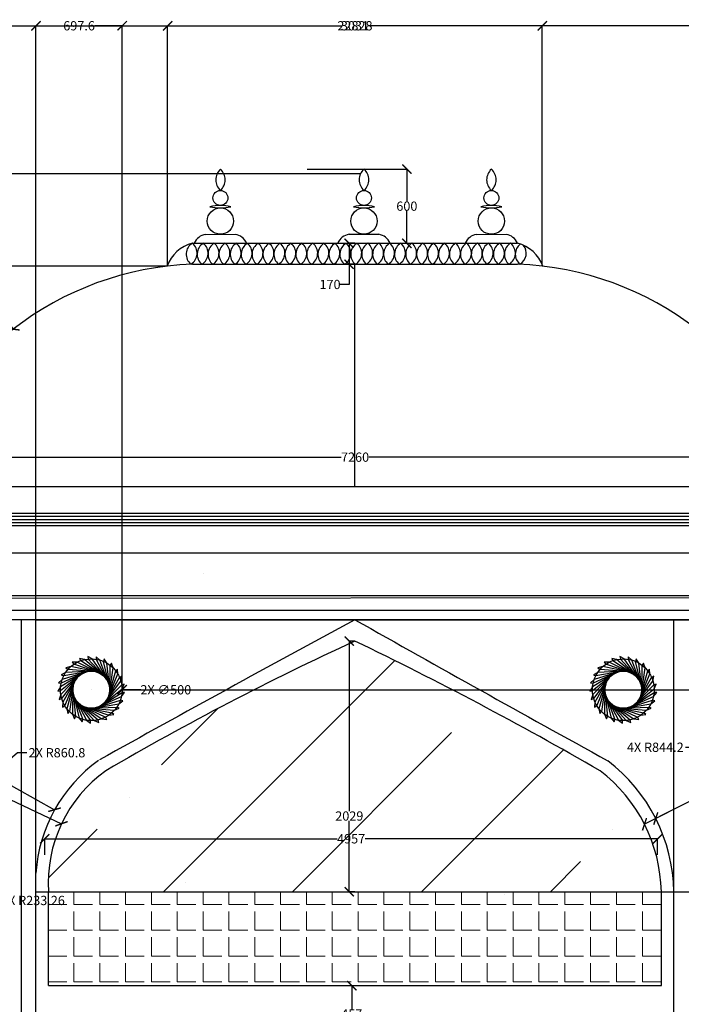
# Model space of a CAD drawing. Units: inches. Extents: x 829 to 33356404, y 1874 to 16983.
# Tile 7 of 9: x 10848 to 16199, y 9014 to 16983. Entities that reach past the tile are written whole.
import ezdxf

# ---------------------------------------------------------------- set-up
doc = ezdxf.new("R2010")
doc.units = ezdxf.units.IN
doc.header["$MEASUREMENT"] = 0
doc.header["$PDMODE"] = 3
for name, color, linetype, lineweight in [('A-ANNO-DIMS', 2, 'Continuous', 18), ('A-ELEV', 7, 'Continuous', 25), ('A-ELEV-PATT', 8, 'Continuous', 13)]:
    doc.layers.add(name, color=color, linetype=linetype, lineweight=lineweight)
doc.styles.get("Standard").update_dxf_attribs({"font": 'arial.ttf'})
doc.dimstyles.get("Standard").update_dxf_attribs({"dimtxt": 75, "dimasz": 75, "dimexe": 0.18, "dimexo": 0.0625, "dimgap": 0.09, "dimtad": 0, "dimtih": 1, "dimtoh": 1, "dimdec": 0, "dimzin": 0, "dimdsep": 46, "dimtxsty": 'Standard', "dimblk": 'ARCHTICK', "dimcen": 0.09, "dimadec": 0, "dimazin": 0, "dimtfac": 1, "dimtdec": 0, "dimtofl": 0, "dimtmove": 0, "dimatfit": 3, "dimfxl": 1, "dimtolj": 1, "dimtzin": 0, "dimarcsym": 0})

# ---------------------------------------------------------------- blocks, each defined once
blk = doc.blocks.new('_ArchTick')
at = {"color": 0, "linetype": 'ByBlock', "const_width": 0.15}
blk.add_lwpolyline([(-0.5, -0.5), (0.5, 0.5)], dxfattribs=at)
blk = doc.blocks.new('*D22')
at = {"layer": 'A-ANNO-DIMS', "color": 0, "lineweight": -2, "transparency": 16777216}
for p, q in [((13559.7, 11954.5), (13513.9, 11954.5)), ((13514.1, 11954.5), (13514.1, 10576.7)), ((13514.1, 9925.5), (13514.1, 10500)), ((13559.7, 9925.5), (13513.9, 9925.5))]:
    blk.add_line(p, q, dxfattribs=at)
at = {"layer": 'Defpoints', "color": 0, "transparency": 16777216}
for p in [(13514.1, 11954.5), (13559.8, 11954.5), (13559.8, 9925.5)]:
    blk.add_point(p, dxfattribs=at)
at = {"layer": 'A-ANNO-DIMS', "color": 0, "lineweight": -2, "transparency": 16777216, "xscale": 75, "yscale": 75, "zscale": 75}
for p, rotation in [((13514.1, 11954.5), 90), ((13514.1, 9925.5), 270)]:
    blk.add_blockref('_ArchTick', p, dxfattribs=dict(at, rotation=rotation))
at = {"layer": 'A-ANNO-DIMS', "color": 0, "transparency": 16777216, "insert": (13514.1, 10538.4), "char_height": 75, "attachment_point": 5}
blk.add_mtext('\\A1;2029', dxfattribs=at)
blk = doc.blocks.new('*D23')
at = {"layer": 'A-ANNO-DIMS', "color": 0, "lineweight": -2, "transparency": 16777216}
for p, q in [((11050.4, 10222.8), (11050.4, 10354.2)), ((11050.4, 10354), (13415.3, 10354)), ((16007.4, 10354), (13642.4, 10354)), ((16007.4, 10222.8), (16007.4, 10354.2))]:
    blk.add_line(p, q, dxfattribs=at)
at = {"layer": 'Defpoints', "color": 0, "transparency": 16777216}
for p in [(16007.4, 10354), (11050.4, 10222.7), (16007.4, 10222.7)]:
    blk.add_point(p, dxfattribs=at)
at = {"layer": 'A-ANNO-DIMS', "color": 0, "lineweight": -2, "transparency": 16777216, "xscale": 75, "yscale": 75, "zscale": 75, "rotation": 180}
blk.add_blockref('_ArchTick', (11050.4, 10354), dxfattribs=at)
at = {"layer": 'A-ANNO-DIMS', "color": 0, "lineweight": -2, "transparency": 16777216, "xscale": 75, "yscale": 75, "zscale": 75}
blk.add_blockref('_ArchTick', (16007.4, 10354), dxfattribs=at)
at = {"layer": 'A-ANNO-DIMS', "color": 0, "transparency": 16777216, "insert": (13528.9, 10354), "char_height": 75, "attachment_point": 5}
blk.add_mtext('\\A1;4957', dxfattribs=at)
blk = doc.blocks.new('*D24')
at = {"layer": 'A-ANNO-DIMS', "color": 0, "lineweight": -2, "transparency": 16777216}
for p, q in [((13534.6, 9165.5), (13534.3, 9165.5)), ((13534.5, 9165.5), (13534.5, 8975.2)), ((13534.5, 8708.5), (13534.5, 8898.7)), ((13534.6, 8708.5), (13534.3, 8708.5))]:
    blk.add_line(p, q, dxfattribs=at)
at = {"layer": 'Defpoints', "color": 0, "transparency": 16777216}
for p in [(13534.7, 9165.5), (13534.5, 8708.5), (13534.7, 8708.5)]:
    blk.add_point(p, dxfattribs=at)
at = {"layer": 'A-ANNO-DIMS', "color": 0, "lineweight": -2, "transparency": 16777216, "xscale": 75, "yscale": 75, "zscale": 75}
for p, rotation in [((13534.5, 9165.5), 90), ((13534.5, 8708.5), 270)]:
    blk.add_blockref('_ArchTick', p, dxfattribs=dict(at, rotation=rotation))
at = {"layer": 'A-ANNO-DIMS', "color": 0, "transparency": 16777216, "insert": (13534.5, 8937), "char_height": 75, "attachment_point": 5}
blk.add_mtext('\\A1;457', dxfattribs=at)
blk = doc.blocks.new('*D55')
at = {"layer": 'A-ANNO-DIMS', "color": 0, "lineweight": -2, "transparency": 16777216}
for p, q in [((9930.8, 13204.1), (9930.8, 13443)), ((9930.8, 13442.8), (13449.1, 13442.8)), ((17190.8, 13442.8), (13672.4, 13442.8)), ((17190.8, 13204.1), (17190.8, 13443))]:
    blk.add_line(p, q, dxfattribs=at)
at = {"layer": 'Defpoints', "color": 0, "transparency": 16777216}
for p in [(17190.8, 13442.8), (9930.8, 13204), (17190.8, 13204)]:
    blk.add_point(p, dxfattribs=at)
at = {"layer": 'A-ANNO-DIMS', "color": 0, "lineweight": -2, "transparency": 16777216, "xscale": 75, "yscale": 75, "zscale": 75, "rotation": 180}
blk.add_blockref('_ArchTick', (9930.8, 13442.8), dxfattribs=at)
at = {"layer": 'A-ANNO-DIMS', "color": 0, "lineweight": -2, "transparency": 16777216, "xscale": 75, "yscale": 75, "zscale": 75}
blk.add_blockref('_ArchTick', (17190.8, 13442.8), dxfattribs=at)
at = {"layer": 'A-ANNO-DIMS', "color": 0, "transparency": 16777216, "insert": (13560.8, 13442.8), "char_height": 75, "attachment_point": 5}
blk.add_mtext('\\A1;7260', dxfattribs=at)
blk = doc.blocks.new('*D56')
at = {"layer": 'A-ANNO-DIMS', "color": 0, "lineweight": -2, "transparency": 16777216}
for p, q in [((13559.7, 15174), (13512.5, 15174)), ((13512.7, 15174), (13512.7, 15004)), ((13559.7, 15004), (13512.5, 15004)), ((13512.7, 15004), (13512.7, 14840.3)), ((13512.7, 14840.3), (13437.7, 14840.3))]:
    blk.add_line(p, q, dxfattribs=at)
at = {"layer": 'Defpoints', "color": 0, "transparency": 16777216}
for p in [(13559.8, 15174), (13512.7, 15004), (13559.8, 15004)]:
    blk.add_point(p, dxfattribs=at)
at = {"layer": 'A-ANNO-DIMS', "color": 0, "lineweight": -2, "transparency": 16777216, "xscale": 75, "yscale": 75, "zscale": 75}
for p, rotation in [((13512.7, 15174), 90), ((13512.7, 15004), 270)]:
    blk.add_blockref('_ArchTick', p, dxfattribs=dict(at, rotation=rotation))
at = {"layer": 'A-ANNO-DIMS', "color": 0, "transparency": 16777216, "insert": (13358.4, 14840.3), "char_height": 75, "attachment_point": 5}
blk.add_mtext('\\A1;170', dxfattribs=at)
blk = doc.blocks.new('*D67')
at = {"layer": 'A-ANNO-DIMS', "color": 0, "lineweight": -2, "transparency": 16777216}
for p, q in [((13174.2, 15774), (13979.7, 15774)), ((13979.5, 15774), (13979.5, 15512.4)), ((13979.5, 15174), (13979.5, 15435.6)), ((13174.2, 15174), (13979.7, 15174))]:
    blk.add_line(p, q, dxfattribs=at)
at = {"layer": 'Defpoints', "color": 0, "transparency": 16777216}
for p in [(13174.2, 15774), (13979.5, 15774), (13174.2, 15174)]:
    blk.add_point(p, dxfattribs=at)
at = {"layer": 'A-ANNO-DIMS', "color": 0, "lineweight": -2, "transparency": 16777216, "xscale": 75, "yscale": 75, "zscale": 75}
for p, rotation in [((13979.5, 15774), 90), ((13979.5, 15174), 270)]:
    blk.add_blockref('_ArchTick', p, dxfattribs=dict(at, rotation=rotation))
at = {"layer": 'A-ANNO-DIMS', "color": 0, "transparency": 16777216, "insert": (13979.5, 15474), "char_height": 75, "attachment_point": 5}
blk.add_mtext('\\A1;600', dxfattribs=at)
blk = doc.blocks.new('*D82')
at = {"layer": 'A-ANNO-DIMS', "color": 0, "lineweight": -2, "transparency": 16777216}
for p, q in [((2145.7, 12292.3), (2145.7, 16934.2)), ((2145.7, 16934), (13417.9, 16934)), ((24973.9, 16934), (13701.7, 16934)), ((24973.9, 12320.9), (24973.9, 16934.2))]:
    blk.add_line(p, q, dxfattribs=at)
at = {"layer": 'Defpoints', "color": 0, "transparency": 16777216}
for p in [(24973.9, 16934), (2145.7, 12292.2), (24973.9, 12320.9)]:
    blk.add_point(p, dxfattribs=at)
at = {"layer": 'A-ANNO-DIMS', "color": 0, "lineweight": -2, "transparency": 16777216, "xscale": 75, "yscale": 75, "zscale": 75, "rotation": 180}
blk.add_blockref('_ArchTick', (2145.7, 16934), dxfattribs=at)
at = {"layer": 'A-ANNO-DIMS', "color": 0, "lineweight": -2, "transparency": 16777216, "xscale": 75, "yscale": 75, "zscale": 75}
blk.add_blockref('_ArchTick', (24973.9, 16934), dxfattribs=at)
at = {"layer": 'A-ANNO-DIMS', "color": 0, "transparency": 16777216, "insert": (13559.8, 16934), "char_height": 75, "attachment_point": 5}
blk.add_mtext('\\A1;22828', dxfattribs=at)
blk = doc.blocks.new('*D83')
at = {"layer": 'A-ANNO-DIMS', "color": 0, "lineweight": -2, "transparency": 16777216}
for p, q in [((13604.5, 15734.9), (985.4, 15734.9)), ((985.6, 15734.9), (985.6, 10279.1)), ((985.6, 4746.5), (985.6, 10202.3)), ((3169.7, 4746.5), (985.4, 4746.5))]:
    blk.add_line(p, q, dxfattribs=at)
at = {"layer": 'Defpoints', "color": 0, "transparency": 16777216}
for p in [(985.6, 15734.9), (13604.5, 15734.9), (3169.8, 4746.5)]:
    blk.add_point(p, dxfattribs=at)
at = {"layer": 'A-ANNO-DIMS', "color": 0, "lineweight": -2, "transparency": 16777216, "xscale": 75, "yscale": 75, "zscale": 75}
for p, rotation in [((985.6, 15734.9), 90), ((985.6, 4746.5), 270)]:
    blk.add_blockref('_ArchTick', p, dxfattribs=dict(at, rotation=rotation))
at = {"layer": 'A-ANNO-DIMS', "color": 0, "transparency": 16777216, "insert": (985.6, 10240.7), "char_height": 75, "attachment_point": 5}
blk.add_mtext('\\A1;10988', dxfattribs=at)
blk = doc.blocks.new('*D84')
at = {"layer": 'A-ANNO-DIMS', "color": 0, "lineweight": -2, "transparency": 16777216}
for p, q in [((12044.3, 14988.9), (985.4, 14988.9)), ((985.6, 14988.9), (985.6, 14134.8)), ((985.6, 13204), (985.6, 14058.1)), ((9930.7, 13204), (985.4, 13204))]:
    blk.add_line(p, q, dxfattribs=at)
at = {"layer": 'Defpoints', "color": 0, "transparency": 16777216}
for p in [(985.6, 14988.9), (12044.4, 14988.9), (9930.8, 13204)]:
    blk.add_point(p, dxfattribs=at)
at = {"layer": 'A-ANNO-DIMS', "color": 0, "lineweight": -2, "transparency": 16777216, "xscale": 75, "yscale": 75, "zscale": 75}
for p, rotation in [((985.6, 14988.9), 90), ((985.6, 13204), 270)]:
    blk.add_blockref('_ArchTick', p, dxfattribs=dict(at, rotation=rotation))
at = {"layer": 'A-ANNO-DIMS', "color": 0, "transparency": 16777216, "insert": (985.6, 14096.5), "char_height": 75, "attachment_point": 5}
blk.add_mtext('\\A1;1785', dxfattribs=at)
blk = doc.blocks.new('*D85')
at = {"layer": 'A-ANNO-DIMS', "color": 0, "lineweight": -2, "transparency": 16777216}
for p, q in [((12044.4, 14989), (12044.4, 16934.2)), ((12044.4, 16934), (13455, 16934)), ((15075.2, 16934), (13664.6, 16934)), ((15075.2, 14989), (15075.2, 16934.2))]:
    blk.add_line(p, q, dxfattribs=at)
at = {"layer": 'Defpoints', "color": 0, "transparency": 16777216}
for p in [(15075.2, 16934), (12044.4, 14988.9), (15075.2, 14988.9)]:
    blk.add_point(p, dxfattribs=at)
at = {"layer": 'A-ANNO-DIMS', "color": 0, "lineweight": -2, "transparency": 16777216, "xscale": 75, "yscale": 75, "zscale": 75, "rotation": 180}
blk.add_blockref('_ArchTick', (12044.4, 16934), dxfattribs=at)
at = {"layer": 'A-ANNO-DIMS', "color": 0, "lineweight": -2, "transparency": 16777216, "xscale": 75, "yscale": 75, "zscale": 75}
blk.add_blockref('_ArchTick', (15075.2, 16934), dxfattribs=at)
at = {"layer": 'A-ANNO-DIMS', "color": 0, "transparency": 16777216, "insert": (13559.8, 16934), "char_height": 75, "attachment_point": 5}
blk.add_mtext('\\A1;3031', dxfattribs=at)
blk = doc.blocks.new('*D91')
at = {"layer": 'A-ANNO-DIMS', "color": 0, "lineweight": -2, "transparency": 16777216}
for p, q in [((11081.8, 9925.5), (26134.1, 9925.5)), ((26133.9, 9925.5), (26133.9, 9354.7)), ((26133.9, 8708.5), (26133.9, 9279.2)), ((11081.8, 8708.5), (26134.1, 8708.5))]:
    blk.add_line(p, q, dxfattribs=at)
at = {"layer": 'Defpoints', "color": 0, "transparency": 16777216}
for p in [(11081.8, 9925.5), (11081.8, 8708.5), (26133.9, 8708.5)]:
    blk.add_point(p, dxfattribs=at)
at = {"layer": 'A-ANNO-DIMS', "color": 0, "lineweight": -2, "transparency": 16777216, "xscale": 75, "yscale": 75, "zscale": 75}
for p, rotation in [((26133.9, 9925.5), 90), ((26133.9, 8708.5), 270)]:
    blk.add_blockref('_ArchTick', p, dxfattribs=dict(at, rotation=rotation))
at = {"layer": 'A-ANNO-DIMS', "color": 0, "transparency": 16777216, "insert": (26133.9, 9317), "char_height": 75, "attachment_point": 5}
blk.add_mtext('\\A1;1217', dxfattribs=at)
blk = doc.blocks.new('*D92')
at = {"layer": 'A-ANNO-DIMS', "color": 0, "lineweight": -2, "transparency": 16777216}
for p, q in [((10979.8, 12127.3), (10979.8, 16934.2)), ((10979.8, 16934), (11201.8, 16934)), ((11677.4, 16934), (11455.4, 16934)), ((11677.4, 11560.1), (11677.4, 16934.2))]:
    blk.add_line(p, q, dxfattribs=at)
at = {"layer": 'Defpoints', "color": 0, "transparency": 16777216}
for p in [(11677.4, 16934), (10979.8, 12127.2), (11677.4, 11560.1)]:
    blk.add_point(p, dxfattribs=at)
at = {"layer": 'A-ANNO-DIMS', "color": 0, "lineweight": -2, "transparency": 16777216, "xscale": 75, "yscale": 75, "zscale": 75, "rotation": 180}
blk.add_blockref('_ArchTick', (10979.8, 16934), dxfattribs=at)
at = {"layer": 'A-ANNO-DIMS', "color": 0, "lineweight": -2, "transparency": 16777216, "xscale": 75, "yscale": 75, "zscale": 75}
blk.add_blockref('_ArchTick', (11677.4, 16934), dxfattribs=at)
at = {"layer": 'A-ANNO-DIMS', "color": 0, "transparency": 16777216, "insert": (11328.6, 16934), "char_height": 75, "attachment_point": 5}
blk.add_mtext('\\A1;697.6', dxfattribs=at)
blk = doc.blocks.new('*D93')
at = {"layer": 'A-ANNO-DIMS', "color": 0, "lineweight": -2, "transparency": 16777216}
for p, q in [((10979.8, 12127.2), (26134.1, 12127.2)), ((26133.9, 12127.2), (26133.9, 11882)), ((26133.9, 11560.1), (26133.9, 11805.3)), ((11677.4, 11560.1), (26134.1, 11560.1))]:
    blk.add_line(p, q, dxfattribs=at)
at = {"layer": 'Defpoints', "color": 0, "transparency": 16777216}
for p in [(10979.8, 12127.2), (11677.4, 11560.1), (26133.9, 11560.1)]:
    blk.add_point(p, dxfattribs=at)
at = {"layer": 'A-ANNO-DIMS', "color": 0, "lineweight": -2, "transparency": 16777216, "xscale": 75, "yscale": 75, "zscale": 75}
for p, rotation in [((26133.9, 12127.2), 90), ((26133.9, 11560.1), 270)]:
    blk.add_blockref('_ArchTick', p, dxfattribs=dict(at, rotation=rotation))
at = {"layer": 'A-ANNO-DIMS', "color": 0, "transparency": 16777216, "insert": (26133.9, 11843.6), "char_height": 75, "attachment_point": 5}
blk.add_mtext('\\A1;567.1', dxfattribs=at)
blk = doc.blocks.new('*D109')
at = {"layer": 'A-ANNO-DIMS', "color": 0, "lineweight": -2, "transparency": 16777216}
for p, q in [((9798.3, 15665.5), (9873.3, 15665.5)), ((9873.3, 15665.5), (10796, 14478.3)), ((12333.6, 12499.6), (12333.8, 12499.6)), ((12333.7, 12499.5), (12333.7, 12499.7))]:
    blk.add_line(p, q, dxfattribs=at)
at = {"layer": 'Defpoints', "color": 0, "transparency": 16777216}
for p in [(10796, 14478.3), (12333.7, 12499.6)]:
    blk.add_point(p, dxfattribs=at)
at = {"layer": 'A-ANNO-DIMS', "color": 0, "lineweight": -2, "transparency": 16777216, "xscale": 75, "yscale": 75, "zscale": 75, "rotation": 307.8527471709181}
blk.add_blockref('_ArchTick', (10796, 14478.3), dxfattribs=at)
at = {"layer": 'A-ANNO-DIMS', "color": 0, "transparency": 16777216, "insert": (9569.2, 15665.5), "char_height": 75, "attachment_point": 5}
blk.add_mtext('\\A1;2X R2506', dxfattribs=at)
blk = doc.blocks.new('*D123')
at = {"layer": 'A-ANNO-DIMS', "color": 0, "lineweight": -2, "transparency": 16777216}
for p, q in [((10418.6, 10943.5), (10493.6, 10943.5)), ((10493.6, 10943.5), (11130.3, 10589.5)), ((12191.3, 9999.5), (12191.5, 9999.5)), ((12191.4, 9999.4), (12191.4, 9999.6))]:
    blk.add_line(p, q, dxfattribs=at)
at = {"layer": 'Defpoints', "color": 0, "transparency": 16777216}
for p in [(11130.3, 10589.5), (12191.4, 9999.5)]:
    blk.add_point(p, dxfattribs=at)
at = {"layer": 'A-ANNO-DIMS', "color": 0, "lineweight": -2, "transparency": 16777216, "xscale": 75, "yscale": 75, "zscale": 75, "rotation": 330.9254937916661}
blk.add_blockref('_ArchTick', (11130.3, 10589.5), dxfattribs=at)
at = {"layer": 'A-ANNO-DIMS', "color": 0, "transparency": 16777216, "insert": (10270.8, 10943.5), "char_height": 75, "attachment_point": 5}
blk.add_mtext('\\A1;R1214', dxfattribs=at)
blk = doc.blocks.new('*D124')
at = {"layer": 'A-ANNO-DIMS', "color": 0, "lineweight": -2, "transparency": 16777216}
for p, q in [((10508.3, 10761.1), (10583.3, 10761.1)), ((10583.3, 10761.1), (11186.3, 10475.5)), ((12191.3, 9999.5), (12191.5, 9999.5)), ((12191.4, 9999.4), (12191.4, 9999.6))]:
    blk.add_line(p, q, dxfattribs=at)
at = {"layer": 'Defpoints', "color": 0, "transparency": 16777216}
for p in [(11186.3, 10475.5), (12191.4, 9999.5)]:
    blk.add_point(p, dxfattribs=at)
at = {"layer": 'A-ANNO-DIMS', "color": 0, "lineweight": -2, "transparency": 16777216, "xscale": 75, "yscale": 75, "zscale": 75, "rotation": 334.6586083454434}
blk.add_blockref('_ArchTick', (11186.3, 10475.5), dxfattribs=at)
at = {"layer": 'A-ANNO-DIMS', "color": 0, "transparency": 16777216, "insert": (10323.9, 10761.1), "char_height": 75, "attachment_point": 5}
blk.add_mtext('\\A1;R1112.1', dxfattribs=at)
blk = doc.blocks.new('*D125')
at = {"layer": 'A-ANNO-DIMS', "color": 0, "lineweight": -2, "transparency": 16777216}
for p, q in [((16724.8, 10888.3), (15992.6, 10517.8)), ((16799.8, 10888.3), (16724.8, 10888.3)), ((14772.3, 9900.1), (14772.5, 9900.1)), ((14772.4, 9900), (14772.4, 9900.2))]:
    blk.add_line(p, q, dxfattribs=at)
at = {"layer": 'Defpoints', "color": 0, "transparency": 16777216}
for p in [(15992.6, 10517.8), (14772.4, 9900.1)]:
    blk.add_point(p, dxfattribs=at)
at = {"layer": 'A-ANNO-DIMS', "color": 0, "lineweight": -2, "transparency": 16777216, "xscale": 75, "yscale": 75, "zscale": 75, "rotation": 206.8466405163161}
blk.add_blockref('_ArchTick', (15992.6, 10517.8), dxfattribs=at)
at = {"layer": 'A-ANNO-DIMS', "color": 0, "transparency": 16777216, "insert": (16991.4, 10888.3), "char_height": 75, "attachment_point": 5}
blk.add_mtext('\\A1;R1367.6', dxfattribs=at)
blk = doc.blocks.new('*D126')
at = {"layer": 'A-ANNO-DIMS', "color": 0, "lineweight": -2, "transparency": 16777216}
for p, q in [((16579.1, 10814.6), (15901.6, 10471.7)), ((16654.1, 10814.6), (16579.1, 10814.6)), ((14772.3, 9900.1), (14772.5, 9900.1)), ((14772.4, 9900), (14772.4, 9900.2))]:
    blk.add_line(p, q, dxfattribs=at)
at = {"layer": 'Defpoints', "color": 0, "transparency": 16777216}
for p in [(15901.6, 10471.7), (14772.4, 9900.1)]:
    blk.add_point(p, dxfattribs=at)
at = {"layer": 'A-ANNO-DIMS', "color": 0, "lineweight": -2, "transparency": 16777216, "xscale": 75, "yscale": 75, "zscale": 75, "rotation": 206.8466187545911}
blk.add_blockref('_ArchTick', (15901.6, 10471.7), dxfattribs=at)
at = {"layer": 'A-ANNO-DIMS', "color": 0, "transparency": 16777216, "insert": (16845.8, 10814.6), "char_height": 75, "attachment_point": 5}
blk.add_mtext('\\A1;R1265.6', dxfattribs=at)
blk = doc.blocks.new('*D127')
at = {"layer": 'A-ANNO-DIMS', "color": 0, "lineweight": -2, "transparency": 16777216}
for p, q in [((11427.3, 11560.1), (11427.5, 11560.1)), ((11427.4, 11560), (11427.4, 11560.2)), ((11827.4, 11560.1), (11677.4, 11560.1))]:
    blk.add_line(p, q, dxfattribs=at)
at = {"layer": 'Defpoints', "color": 0, "transparency": 16777216}
for p in [(11177.4, 11560.1), (11677.4, 11560.1)]:
    blk.add_point(p, dxfattribs=at)
at = {"layer": 'A-ANNO-DIMS', "color": 0, "lineweight": -2, "transparency": 16777216, "xscale": 75, "yscale": 75, "zscale": 75, "rotation": 180.0000873187677}
blk.add_blockref('_ArchTick', (11677.4, 11560.1), dxfattribs=at)
at = {"layer": 'A-ANNO-DIMS', "color": 0, "transparency": 16777216, "insert": (12030.2, 11560.1), "char_height": 75, "attachment_point": 5}
blk.add_mtext('\\A1;2X ∅500', dxfattribs=at)
blk = doc.blocks.new('*D129')
at = {"layer": 'A-ANNO-DIMS', "color": 0, "lineweight": -2, "transparency": 16777216}
for p, q in [((10830.9, 11050.5), (10439.6, 10713.3)), ((10905.9, 11050.5), (10830.9, 11050.5)), ((9787.3, 10151.5), (9787.5, 10151.5)), ((9787.4, 10151.4), (9787.4, 10151.6))]:
    blk.add_line(p, q, dxfattribs=at)
at = {"layer": 'Defpoints', "color": 0, "transparency": 16777216}
for p in [(10439.6, 10713.3), (9787.4, 10151.5)]:
    blk.add_point(p, dxfattribs=at)
at = {"layer": 'A-ANNO-DIMS', "color": 0, "lineweight": -2, "transparency": 16777216, "xscale": 75, "yscale": 75, "zscale": 75, "rotation": 220.7456490042762}
blk.add_blockref('_ArchTick', (10439.6, 10713.3), dxfattribs=at)
at = {"layer": 'A-ANNO-DIMS', "color": 0, "transparency": 16777216, "insert": (11149.7, 11050.5), "char_height": 75, "attachment_point": 5}
blk.add_mtext('\\A1;2X R860.8', dxfattribs=at)
blk = doc.blocks.new('*D130')
at = {"layer": 'A-ANNO-DIMS', "color": 0, "lineweight": -2, "transparency": 16777216}
for p, q in [((16233.3, 11094.9), (16308.3, 11094.9)), ((16308.3, 11094.9), (16682.6, 10753.6)), ((17306.3, 10184.7), (17306.5, 10184.7)), ((17306.4, 10184.6), (17306.4, 10184.8))]:
    blk.add_line(p, q, dxfattribs=at)
at = {"layer": 'Defpoints', "color": 0, "transparency": 16777216}
for p in [(16682.6, 10753.6), (17306.4, 10184.7)]:
    blk.add_point(p, dxfattribs=at)
at = {"layer": 'A-ANNO-DIMS', "color": 0, "lineweight": -2, "transparency": 16777216, "xscale": 75, "yscale": 75, "zscale": 75, "rotation": 317.6357309782866}
blk.add_blockref('_ArchTick', (16682.6, 10753.6), dxfattribs=at)
at = {"layer": 'A-ANNO-DIMS', "color": 0, "transparency": 16777216, "insert": (15989.1, 11094.9), "char_height": 75, "attachment_point": 5}
blk.add_mtext('\\A1;4X R844.2', dxfattribs=at)
blk = doc.blocks.new('*D134')
at = {"layer": 'A-ANNO-DIMS', "color": 0, "lineweight": -2, "transparency": 16777216}
for p, q in [((10607.7, 9854.8), (10543.8, 9719.1)), ((10682.7, 9854.8), (10607.7, 9854.8)), ((10444.4, 9508.1), (10444.5, 9508.1)), ((10444.5, 9508), (10444.5, 9508.2))]:
    blk.add_line(p, q, dxfattribs=at)
at = {"layer": 'Defpoints', "color": 0, "transparency": 16777216}
for p in [(10543.8, 9719.1), (10444.5, 9508.1)]:
    blk.add_point(p, dxfattribs=at)
at = {"layer": 'A-ANNO-DIMS', "color": 0, "lineweight": -2, "transparency": 16777216, "xscale": 75, "yscale": 75, "zscale": 75, "rotation": 244.7886305373675}
blk.add_blockref('_ArchTick', (10543.8, 9719.1), dxfattribs=at)
at = {"layer": 'A-ANNO-DIMS', "color": 0, "transparency": 16777216, "insert": (10955.6, 9854.8), "char_height": 75, "attachment_point": 5}
blk.add_mtext('\\A1;2X R233.26', dxfattribs=at)

msp = doc.modelspace()

# ---------------------------------------------------------------- hatches: boundary and pattern name
at = {"layer": 'A-ELEV-PATT'}
h = msp.add_hatch(dxfattribs=at)
h.set_pattern_fill('ANSI35', color=256, scale=5900)
h.paths.add_polyline_path([(13559.778, 11954.468, 0.02477271), (11545.586, 10904.83, 0.26007445), (11081.778, 9925.468), (16037.778, 9925.468, 0.22810939), (15542.066, 10904.83, 0.01846983)])
h.paths.add_polyline_path([(13379.549, 10460.544), (13650.132, 10460.544), (13650.132, 10615.097), (13379.549, 10615.097)], flags=24)
h.paths.add_polyline_path([(13395.284, 10276.184), (13665.867, 10276.184), (13665.867, 10430.737), (13395.284, 10430.737)], flags=24)
h = msp.add_hatch(dxfattribs=at)
h.set_pattern_fill('ANGLE', color=256, scale=760)
h.set_pattern_definition([(0, (0, 0), (0, 209), [152, -57]), (90, (0, 0), (-209, 1e-14), [152, -57])])
h.paths.add_polyline_path([(11081.778, 9925.468), (11081.778, 9165.468), (16037.778, 9165.468), (16037.778, 9925.468)])

# ---------------------------------------------------------------- linework, layer by layer
at = {"layer": 'A-ELEV'}
for p, q in [((12351.34, 15245.971), (12591.591, 15247.24)), ((13512.395, 15246.139), (13752.646, 15247.408)), ((14542.78, 15245.971), (14783.031, 15247.24)), ((12244.919, 15174.032), (14874.638, 15174.032)), ((12244.919, 15004.032), (14874.638, 15004.032)), ((13559.778, 13204.032), (13559.778, 15004.032)), ((3169.778, 13204.032), (23949.778, 13204.032)), ((23949.778, 12986.532), (3169.778, 12986.532)), ((23949.778, 12961.532), (3169.778, 12961.532)), ((23949.778, 12936.532), (3169.778, 12936.532)), ((23949.778, 12911.532), (3169.778, 12911.532)), ((23949.778, 12886.532), (3169.778, 12886.532)), ((3169.778, 12669.032), (23949.778, 12669.032)), ((24973.929, 12320.882), (2145.628, 12320.882)), ((24973.929, 12310.744), (2145.651, 12292.214)), ((22522.278, 12202.212), (3169.778, 12202.212)), ((18091.883, 12127.212), (9559.826, 12127.212)), ((10860.89, 12127.212), (10860.89, 5024.468)), ((10979.778, 5024.468), (10979.778, 12127.212)), ((16139.778, 5660.468), (16139.778, 12127.212)), ((11372.313, 11803.932), (11333.24, 11813.935)), ((11333.24, 11813.935), (11342.184, 11795.107)), ((11515.543, 11681.423), (11342.184, 11795.107)), ((11530.058, 11669.416), (11372.313, 11803.932)), ((11434.689, 11809.964), (11399.331, 11829.37)), ((11399.331, 11829.37), (11403.312, 11808.91)), ((11542.953, 11655.684), (11403.312, 11808.91)), ((11554.025, 11640.445), (11434.689, 11809.964)), ((11467.184, 11827.883), (11465.951, 11807.077)), ((11563.1, 11623.938), (11465.951, 11807.077)), ((11496.605, 11800.294), (11467.184, 11827.883)), ((11570.034, 11606.423), (11496.605, 11800.294)), ((11532.536, 11809.57), (11526.167, 11789.723)), ((11554.171, 11775.53), (11532.536, 11809.57)), ((15675.192, 11803.932), (15636.119, 11813.935)), ((15636.119, 11813.935), (15645.063, 11795.107)), ((15818.422, 11681.423), (15645.063, 11795.107)), ((15832.937, 11669.416), (15675.192, 11803.932)), ((15737.568, 11809.964), (15702.21, 11829.37)), ((15702.21, 11829.37), (15706.19, 11808.91)), ((15845.832, 11655.684), (15706.19, 11808.91)), ((15856.904, 11640.445), (15737.568, 11809.964)), ((15770.063, 11827.883), (15768.83, 11807.077)), ((15865.979, 11623.938), (15768.83, 11807.077)), ((15799.484, 11800.294), (15770.063, 11827.883)), ((15872.913, 11606.423), (15799.484, 11800.294)), ((15835.415, 11809.57), (15829.046, 11789.723)), ((15857.05, 11775.53), (15835.415, 11809.57)), ((11261.643, 11747.241), (11222.584, 11737.183)), ((11222.584, 11737.183), (11239.492, 11724.993)), ((11446.176, 11708.888), (11239.492, 11724.993)), ((11464.679, 11705.358), (11261.643, 11747.241)), ((11313.398, 11782.577), (11273.064, 11782.548)), ((11273.064, 11782.548), (11286.409, 11766.537)), ((11482.594, 11699.537), (11286.409, 11766.537)), ((11499.639, 11691.517), (11313.398, 11782.577)), ((11574.719, 11588.178), (11526.167, 11789.723)), ((11577.08, 11569.489), (11554.171, 11775.53)), ((11574.719, 11531.963), (11603.77, 11737.228)), ((11577.08, 11550.652), (11580.176, 11757.94)), ((11591.28, 11775.579), (11580.176, 11757.94)), ((11603.77, 11737.228), (11591.28, 11775.579)), ((11639.725, 11728.047), (11624.583, 11713.723)), ((11642.286, 11687.795), (11639.725, 11728.047)), ((15564.522, 11747.241), (15525.463, 11737.183)), ((15525.463, 11737.183), (15542.371, 11724.993)), ((15749.055, 11708.888), (15542.371, 11724.993)), ((15767.558, 11705.358), (15564.522, 11747.241)), ((15616.277, 11782.577), (15575.943, 11782.548)), ((15575.943, 11782.548), (15589.288, 11766.537)), ((15785.473, 11699.537), (15589.288, 11766.537)), ((15802.518, 11691.517), (15616.277, 11782.577)), ((15877.598, 11588.178), (15829.046, 11789.723)), ((15879.959, 11569.489), (15857.05, 11775.53)), ((15877.598, 11531.963), (15906.649, 11737.228)), ((15879.959, 11550.652), (15883.055, 11757.94)), ((15894.159, 11775.579), (15883.055, 11757.94)), ((15906.649, 11737.228), (15894.159, 11775.579)), ((15942.604, 11728.047), (15927.462, 11713.723)), ((15945.165, 11687.795), (15942.604, 11728.047)), ((11191.973, 11644.247), (11162.591, 11616.616)), ((11339.208, 11681.423), (11177.517, 11551.679)), ((11355.113, 11691.517), (11178.435, 11583.06)), ((11324.694, 11669.416), (11180.539, 11520.429)), ((11372.157, 11699.537), (11183.279, 11614.08)), ((11220.303, 11700.145), (11184.972, 11680.689)), ((11184.972, 11680.689), (11204.38, 11673.087)), ((11311.799, 11655.684), (11187.453, 11489.805)), ((11390.072, 11705.358), (11191.973, 11644.247)), ((11300.727, 11640.445), (11198.152, 11460.289)), ((11408.576, 11708.888), (11204.38, 11673.087)), ((11427.376, 11710.071), (11220.303, 11700.145)), ((11554.025, 11479.697), (11656.6, 11659.853)), ((11563.1, 11496.204), (11642.286, 11687.795)), ((11570.034, 11513.718), (11624.583, 11713.723)), ((11674.828, 11669.961), (11656.6, 11659.853)), ((11667.298, 11630.336), (11674.828, 11669.961)), ((15494.852, 11644.247), (15465.47, 11616.616)), ((15642.087, 11681.423), (15480.396, 11551.679)), ((15657.992, 11691.517), (15481.314, 11583.06)), ((15627.573, 11669.416), (15483.418, 11520.429)), ((15675.036, 11699.537), (15486.158, 11614.08)), ((15523.182, 11700.145), (15487.851, 11680.689)), ((15487.851, 11680.689), (15507.259, 11673.087)), ((15614.678, 11655.684), (15490.332, 11489.805)), ((15692.951, 11705.358), (15494.852, 11644.247)), ((15603.605, 11640.445), (15501.031, 11460.289)), ((15711.455, 11708.888), (15507.259, 11673.087)), ((15730.255, 11710.071), (15523.182, 11700.145)), ((15856.904, 11479.697), (15959.478, 11659.853)), ((15865.979, 11496.204), (15945.165, 11687.795)), ((15872.913, 11513.718), (15927.462, 11713.723)), ((15977.707, 11669.961), (15959.478, 11659.853)), ((15970.177, 11630.336), (15977.707, 11669.961)), ((11178.435, 11583.06), (11156.847, 11548.991)), ((11162.591, 11616.616), (11183.279, 11614.08)), ((11291.652, 11623.938), (11212.465, 11432.346)), ((11284.717, 11606.423), (11230.168, 11406.418)), ((11280.033, 11588.178), (11250.981, 11382.913)), ((11277.672, 11569.489), (11274.576, 11362.202)), ((11515.543, 11438.718), (11677.235, 11568.463)), ((11530.058, 11450.725), (11674.213, 11599.712)), ((11542.953, 11464.457), (11667.298, 11630.336)), ((11694.382, 11604.969), (11674.213, 11599.712)), ((11677.235, 11568.463), (11694.382, 11604.969)), ((15481.314, 11583.06), (15459.726, 11548.991)), ((15465.47, 11616.616), (15486.158, 11614.08)), ((15594.531, 11623.938), (15515.344, 11432.346)), ((15587.596, 11606.423), (15533.047, 11406.418)), ((15582.912, 11588.178), (15553.86, 11382.913)), ((15580.551, 11569.489), (15577.455, 11362.202)), ((15818.422, 11438.718), (15980.114, 11568.463)), ((15832.937, 11450.725), (15977.092, 11599.712)), ((15845.832, 11464.457), (15970.177, 11630.336)), ((15997.261, 11604.969), (15977.092, 11599.712)), ((15980.114, 11568.463), (15997.261, 11604.969)), ((11156.847, 11548.991), (11177.517, 11551.679)), ((11180.539, 11520.429), (11168.102, 11482.061)), ((11168.102, 11482.061), (11187.453, 11489.805)), ((11277.672, 11550.652), (11300.58, 11344.611)), ((11280.033, 11531.963), (11328.584, 11330.418)), ((11284.717, 11513.718), (11358.146, 11319.847)), ((11291.652, 11496.204), (11388.8, 11313.065)), ((11300.727, 11479.697), (11420.062, 11310.178)), ((11464.679, 11414.783), (11662.778, 11475.894)), ((11482.594, 11420.604), (11671.472, 11506.061)), ((11499.639, 11428.625), (11676.316, 11537.081)), ((11682.985, 11470.784), (11662.778, 11475.894)), ((11671.472, 11506.061), (11697.16, 11537.157)), ((11697.16, 11537.157), (11676.316, 11537.081)), ((15459.726, 11548.991), (15480.396, 11551.679)), ((15483.418, 11520.429), (15470.981, 11482.061)), ((15470.981, 11482.061), (15490.332, 11489.805)), ((15580.551, 11550.652), (15603.459, 11344.611)), ((15582.912, 11531.963), (15631.463, 11330.418)), ((15587.596, 11513.718), (15661.025, 11319.847)), ((15594.531, 11496.204), (15691.679, 11313.065)), ((15603.605, 11479.697), (15722.941, 11310.178)), ((15767.558, 11414.783), (15965.657, 11475.894)), ((15785.473, 11420.604), (15974.351, 11506.061)), ((15802.518, 11428.625), (15979.195, 11537.081)), ((15985.864, 11470.784), (15965.657, 11475.894)), ((15974.351, 11506.061), (16000.039, 11537.157)), ((16000.039, 11537.157), (15979.195, 11537.081)), ((11198.152, 11460.289), (11195.648, 11420.033)), ((11195.648, 11420.033), (11212.465, 11432.346)), ((11230.168, 11406.418), (11237.754, 11366.804)), ((11311.799, 11464.457), (11451.44, 11311.231)), ((11324.694, 11450.725), (11482.438, 11316.21)), ((11339.208, 11438.718), (11512.568, 11325.034)), ((11355.113, 11428.625), (11541.354, 11337.564)), ((11372.157, 11420.604), (11568.342, 11353.604)), ((11390.072, 11414.783), (11593.108, 11372.9)), ((11408.576, 11411.253), (11615.26, 11395.148)), ((11427.376, 11410.071), (11634.449, 11419.996)), ((11446.176, 11411.253), (11650.372, 11447.054)), ((11615.26, 11395.148), (11652.75, 11410.022)), ((11652.75, 11410.022), (11634.449, 11419.996)), ((11650.372, 11447.054), (11682.985, 11470.784)), ((15501.031, 11460.289), (15498.527, 11420.033)), ((15498.527, 11420.033), (15515.344, 11432.346)), ((15533.047, 11406.418), (15540.633, 11366.804)), ((15614.678, 11464.457), (15754.319, 11311.231)), ((15627.573, 11450.725), (15785.317, 11316.21)), ((15642.087, 11438.718), (15815.447, 11325.034)), ((15657.992, 11428.625), (15844.233, 11337.564)), ((15675.036, 11420.604), (15871.221, 11353.604)), ((15692.951, 11414.783), (15895.987, 11372.9)), ((15711.455, 11411.253), (15918.139, 11395.148)), ((15730.255, 11410.071), (15937.328, 11419.996)), ((15749.055, 11411.253), (15953.251, 11447.054)), ((15918.139, 11395.148), (15955.629, 11410.022)), ((15955.629, 11410.022), (15937.328, 11419.996)), ((15953.251, 11447.054), (15985.864, 11470.784)), ((11237.754, 11366.804), (11250.981, 11382.913)), ((11274.576, 11362.202), (11291.774, 11325.719)), ((11291.774, 11325.719), (11300.58, 11344.611)), ((11328.584, 11330.418), (11354.315, 11299.359)), ((11354.315, 11299.359), (11358.146, 11319.847)), ((11488.951, 11296.41), (11482.438, 11316.21)), ((11512.568, 11325.034), (11552.587, 11320.007)), ((11552.587, 11320.007), (11541.354, 11337.564)), ((11568.342, 11353.604), (11608.354, 11358.688)), ((11608.354, 11358.688), (11593.108, 11372.9)), ((15540.633, 11366.804), (15553.86, 11382.913)), ((15577.455, 11362.202), (15594.653, 11325.719)), ((15594.653, 11325.719), (15603.459, 11344.611)), ((15631.463, 11330.418), (15657.194, 11299.359)), ((15657.194, 11299.359), (15661.025, 11319.847)), ((15791.83, 11296.41), (15785.317, 11316.21)), ((15815.447, 11325.034), (15855.466, 11320.007)), ((15855.466, 11320.007), (15844.233, 11337.564)), ((15871.221, 11353.604), (15911.233, 11358.688)), ((15911.233, 11358.688), (15895.987, 11372.9)), ((11388.8, 11313.065), (11421.447, 11289.38)), ((11421.447, 11289.38), (11420.062, 11310.178)), ((11451.44, 11311.231), (11488.951, 11296.41)), ((15691.679, 11313.065), (15724.326, 11289.38)), ((15724.326, 11289.38), (15722.941, 11310.178)), ((15754.319, 11311.231), (15791.83, 11296.41)), ((10979.778, 9925.468), (16139.778, 9925.468)), ((11081.778, 9165.468), (11081.778, 9925.468)), ((11081.778, 9165.468), (11081.778, 9925.468)), ((16037.778, 9165.468), (16037.778, 9925.468)), ((11081.778, 9165.468), (16037.778, 9165.468))]:
    msp.add_line(p, q, dxfattribs=at)
for points in [[(12471.689, 15601.119, 0.4532599), (12471.689, 15773.038, 0.44427359)], [(13632.744, 15601.287, 0.45110227), (13632.744, 15774.032, 0.4421588)], [(14663.13, 15601.119, 0.4532599), (14663.13, 15773.038, 0.44427359)], [(12386.695, 15469.276, 0.10911966), (12556.695, 15469.373, 0.12713777)], [(13547.75, 15469.445, 0.10911966), (13717.75, 15469.542, 0.12713777)], [(14578.136, 15469.276, 0.10911966), (14748.136, 15469.373, 0.12713777)], [(12233.079, 15004.444, 0.52056705), (12244.919, 15174.032, 0.52056705)], [(12321.864, 15004.032, 0.52056705), (12333.704, 15173.619, 0.52056705)], [(12410.146, 15004.032, 0.52056705), (12421.986, 15173.619, 0.52056705)], [(12498.427, 15004.032, 0.52056705), (12510.267, 15173.619, 0.52056705)], [(12588.919, 15004.032, 0.52056705), (12600.758, 15173.619, 0.52056705)], [(12677.704, 15003.619, 0.52056705), (12689.544, 15173.206, 0.52056705)], [(12765.986, 15003.619, 0.52056705), (12777.825, 15173.206, 0.52056705)], [(12854.267, 15003.619, 0.52056705), (12866.107, 15173.206, 0.52056705)], [(12942.801, 15004.444, 0.52056705), (12954.64, 15174.032, 0.52056705)], [(13031.586, 15004.032, 0.52056705), (13043.426, 15173.619, 0.52056705)], [(13119.868, 15004.032, 0.52056705), (13131.707, 15173.619, 0.52056705)], [(13208.149, 15004.032, 0.52056705), (13219.989, 15173.619, 0.52056705)], [(13298.641, 15004.032, 0.52056705), (13310.48, 15173.619, 0.52056705)], [(13387.426, 15003.619, 0.52056705), (13399.266, 15173.206, 0.52056705)], [(13475.708, 15003.619, 0.52056705), (13487.547, 15173.206, 0.52056705)], [(13563.989, 15003.619, 0.52056705), (13575.829, 15173.206, 0.52056705)], [(13652.523, 15004.682, 0.52056705), (13664.362, 15174.269, 0.52056705)], [(13741.308, 15004.269, 0.52056705), (13753.148, 15173.857, 0.52056705)], [(13829.59, 15004.269, 0.52056705), (13841.429, 15173.857, 0.52056705)], [(13917.871, 15004.269, 0.52056705), (13929.711, 15173.857, 0.52056705)], [(14008.362, 15004.269, 0.52056705), (14020.202, 15173.857, 0.52056705)], [(14097.148, 15003.857, 0.52056705), (14108.987, 15173.444, 0.52056705)], [(14185.429, 15003.857, 0.52056705), (14197.269, 15173.444, 0.52056705)], [(14273.711, 15003.857, 0.52056705), (14285.55, 15173.444, 0.52056705)], [(14362.244, 15004.92, 0.52056705), (14374.084, 15174.507, 0.52056705)], [(14451.03, 15004.507, 0.52056705), (14462.869, 15174.095, 0.52056705)], [(14539.311, 15004.507, 0.52056705), (14551.151, 15174.095, 0.52056705)], [(14627.593, 15004.507, 0.52056705), (14639.432, 15174.095, 0.52056705)], [(14718.084, 15004.507, 0.52056705), (14729.924, 15174.095, 0.52056705)], [(14806.87, 15004.095, 0.52056705), (14818.709, 15173.682, 0.52056705)]]:
    msp.add_lwpolyline(points, format="xyb", close=True, dxfattribs=at)
msp.add_lwpolyline([(14897.331, 15167.109, 0.4852779), (14895.151, 15004.095, 0.44858264), (14923.858, 15156.413)], format="xyb", dxfattribs=at)
for centre, radius in [((12471.689, 15540.625), 60.494), ((13632.744, 15540.793), 60.494), ((14663.13, 15540.625), 60.494), ((12471.465, 15353.328), 106.722), ((13632.52, 15353.496), 106.722), ((14662.906, 15353.328), 106.722), ((11427.376, 11560.071), 250), ((15730.255, 11560.071), 250), ((11427.376, 11560.071), 150), ((15730.255, 11560.071), 150)]:
    msp.add_circle(centre, radius, dxfattribs=at)
for centre, radius, start, end in [((12371.712, 15125.734), 121.951, 99.6167767, 156.6690648), ((12571.218, 15125.734), 121.951, 23.3309352, 80.3832233), ((13532.768, 15125.902), 121.951, 99.6167767, 156.6690648), ((13732.273, 15125.902), 121.951, 23.3309352, 80.3832233), ((14563.153, 15125.734), 121.951, 99.6167767, 156.6690648), ((14762.659, 15125.734), 121.951, 23.3309352, 80.3832233), ((12321.124, 14883.574), 300.288, 104.7010393, 159.5900862), ((14798.432, 14883.574), 300.288, 20.4099138, 75.2989607), ((12333.736, 12499.606), 2506, 92.0310878, 163.6743952), ((14785.821, 12499.606), 2506, 16.3256048, 87.9689122), ((105945.971, -158561.971), 194087.624, 118.42464241, 119.12027495), ((113344.874, 188445.383), 202596.059, 240.49284352, 241.15500731), ((23138.874, -8884.602), 22935.255, 114.6868242, 120.3631498), ((348.291, -15392.637), 30371.163, 59.982149, 64.2146407), ((12191.429, 9999.464), 1214.116, 125.5021837, 176.3487949), ((14772.427, 9900.135), 1367.605, 1.1469428, 52.5463042), ((12191.429, 9999.464), 1112.116, 125.5021837, 183.8150306), ((14772.427, 9900.135), 1265.605, 1.1469428, 52.5463042)]:
    msp.add_arc(centre, radius, start, end, dxfattribs=at)

# ---------------------------------------------------------------- dimensions: what is measured, and where the dimension line sits
at = {"layer": 'A-ANNO-DIMS'}
for base, p1, p2, override, picture, middle in [((24973.929, 16934.032), (2145.651, 12292.214), (24973.929, 12320.882), {"dimdec": 0, "dimlfac": 1, "dimrnd": 0, "dimzin": 0, "dimdsep": 46, "dimlunit": 2}, '*D82', (13559.79, 16934.032)), ((11677.376, 16934.032), (10979.778, 12127.212), (11677.376, 11560.071), {"dimdec": 1, "dimlfac": 1, "dimrnd": 0, "dimzin": 0, "dimdsep": 46, "dimlunit": 2}, '*D92', (11328.577, 16934.032)), ((15075.167, 16934.032), (12044.389, 14988.895), (15075.167, 14988.895), {"dimdec": 0, "dimlfac": 1, "dimrnd": 0, "dimzin": 0, "dimdsep": 46, "dimlunit": 2}, '*D85', (13559.778, 16934.032)), ((17190.778, 13442.842), (9930.778, 13204.032), (17190.778, 13204.032), {"dimclrd": 0, "dimclre": 0, "dimclrt": 0}, '*D55', (13560.778, 13442.842)), ((16007.362, 10353.998), (11050.362, 10222.746), (16007.362, 10222.746), {"dimclrd": 0, "dimclre": 0, "dimclrt": 0}, '*D23', (13528.862, 10353.998))]:
    dim = msp.add_linear_dim(base=base, p1=p1, p2=p2, dimstyle='Standard', override=override, dxfattribs=at)
    dim.commit()
    dim.dimension.update_dxf_attribs({"geometry": picture, "text_midpoint": middle})
for base, p1, p2, override, picture, middle in [((13979.488, 15774.032), (13174.185, 15174.032), (13174.185, 15774.032), {"dimclrd": 0, "dimclre": 0, "dimclrt": 0}, '*D67', (13979.488, 15474.032)), ((985.628, 15734.879), (3169.778, 4746.468), (13604.527, 15734.879), {"dimdec": 0, "dimlfac": 1, "dimrnd": 0, "dimzin": 0, "dimdsep": 46, "dimlunit": 2}, '*D83', (985.628, 10240.673)), ((985.628, 14988.895), (9930.778, 13204.032), (12044.389, 14988.895), {"dimdec": 0, "dimlfac": 1, "dimrnd": 0, "dimzin": 0, "dimdsep": 46, "dimlunit": 2}, '*D84', (985.628, 14096.463)), ((26133.929, 11560.071), (10979.778, 12127.212), (11677.376, 11560.071), {"dimdec": 1, "dimlfac": 1, "dimrnd": 0, "dimzin": 0, "dimdsep": 46, "dimlunit": 2}, '*D93', (26133.929, 11843.641)), ((26133.929, 8708.468), (11081.778, 9925.468), (11081.778, 8708.468), {"dimdec": 0, "dimlfac": 1, "dimrnd": 0, "dimzin": 0, "dimdsep": 46, "dimlunit": 2}, '*D91', (26133.929, 9316.968)), ((13534.477, 8708.468), (13534.687, 9165.468), (13534.687, 8708.468), {"dimclrd": 0, "dimclre": 0, "dimclrt": 0}, '*D24', (13534.477, 8936.968))]:
    dim = msp.add_linear_dim(base=base, p1=p1, p2=p2, angle=90, dimstyle='Standard', override=override, dxfattribs=at)
    dim.commit()
    dim.dimension.update_dxf_attribs({"geometry": picture, "text_midpoint": middle})
for center, mpoint, text, override, picture, middle in [((12333.736, 12499.606), (10795.968, 14478.32), '2X <>', {"dimdec": 0, "dimlfac": 1, "dimrnd": 0, "dimzin": 0, "dimdsep": 46, "dimlunit": 2}, '*D109', (9569.151, 15665.548)), ((9787.406, 10151.495), (10439.564, 10713.344), '2X <>', {"dimdec": 1, "dimlfac": 1, "dimrnd": 0, "dimzin": 0, "dimdsep": 46, "dimlunit": 2}, '*D129', (11149.674, 11050.454)), ((17306.384, 10184.731), (16682.61, 10753.602), '4X <>', {"dimdec": 1, "dimlfac": 1, "dimrnd": 0, "dimzin": 0, "dimdsep": 46, "dimlunit": 2}, '*D130', (15989.122, 11094.924))]:
    dim = msp.add_radius_dim(center=center, mpoint=mpoint, text=text, dimstyle='Standard', override=override, dxfattribs=at)
    dim.commit()
    dim.dimension.update_dxf_attribs({"geometry": picture, "text_midpoint": middle, "dimtype": 164})
for base, p1, p2, picture, middle in [((13512.699, 15004.032), (13559.778, 15174.032), (13559.778, 15004.032), '*D56', (13358.414, 14840.283)), ((13514.073, 11954.468), (13559.778, 9925.468), (13559.778, 11954.468), '*D22', (13514.073, 10538.358))]:
    dim = msp.add_linear_dim(base=base, p1=p1, p2=p2, angle=90, dimstyle='Standard', override={"dimclrd": 0, "dimclre": 0, "dimclrt": 0}, dxfattribs=at)
    dim.commit()
    dim.dimension.update_dxf_attribs({"geometry": picture, "text_midpoint": middle, "dimtype": 160})
dim = msp.add_diameter_dim_2p(p1=(11177.376, 11560.07), p2=(11677.376, 11560.071), text='2X <>', dimstyle='Standard', override={"dimdec": 0, "dimlfac": 1, "dimrnd": 0, "dimzin": 0, "dimdsep": 46, "dimlunit": 2}, dxfattribs=at)
dim.commit()
dim.dimension.update_dxf_attribs({"geometry": '*D127', "text_midpoint": (11827.376, 11560.071)})
for center, mpoint, override, picture, middle in [((12191.429, 9999.464), (11130.306, 10589.459), {"dimdec": 0, "dimlfac": 1, "dimrnd": 0, "dimzin": 0, "dimdsep": 46, "dimlunit": 2}, '*D123', (10270.819, 10943.456)), ((14772.427, 9900.135), (15992.629, 10517.751), {"dimdec": 1, "dimlfac": 1, "dimrnd": 0, "dimzin": 0, "dimdsep": 46, "dimlunit": 2}, '*D125', (16991.382, 10888.321)), ((14772.427, 9900.135), (15901.623, 10471.687), {"dimdec": 1, "dimlfac": 1, "dimrnd": 0, "dimzin": 0, "dimdsep": 46, "dimlunit": 2}, '*D126', (16845.773, 10814.618)), ((12191.429, 9999.464), (11186.329, 10475.461), {"dimdec": 1, "dimlfac": 1, "dimrnd": 0, "dimzin": 0, "dimdsep": 46, "dimlunit": 2}, '*D124', (10323.85, 10761.06))]:
    dim = msp.add_radius_dim(center=center, mpoint=mpoint, dimstyle='Standard', override=override, dxfattribs=at)
    dim.commit()
    dim.dimension.update_dxf_attribs({"geometry": picture, "text_midpoint": middle, "dimtype": 164})
dim = msp.add_radius_dim(center=(10444.455, 9508.068), mpoint=(10543.814, 9719.108), text='2X <>', dimstyle='Standard', override={"dimdec": 2, "dimlfac": 1, "dimrnd": 0, "dimzin": 0, "dimdsep": 46, "dimlunit": 2}, dxfattribs=at)
dim.commit()
dim.dimension.update_dxf_attribs({"geometry": '*D134', "text_midpoint": (10955.555, 9854.819)})

doc.saveas('drawing.dxf')
